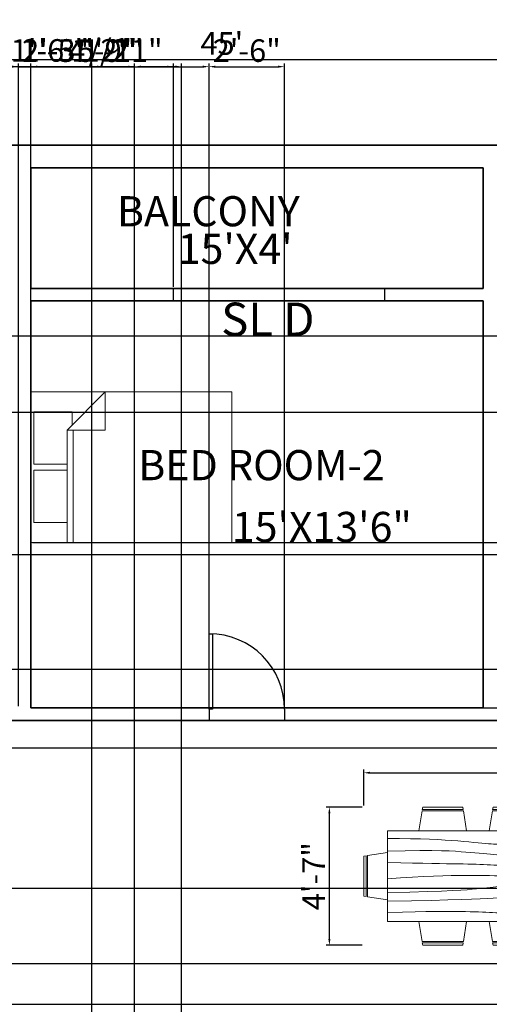
# Model space of a CAD drawing. Units: inches. Extents: x 3542 to 4275, y 1005 to 1722.
# Tile 3 of 6: x 3831 to 4018, y 1330 to 1722. Entities that reach past the tile are written whole.
import ezdxf

# ---------------------------------------------------------------- set-up
doc = ezdxf.new("R2010")
doc.units = ezdxf.units.IN
doc.layers.get('0').update_dxf_attribs({"color": 211})
for name, color, linetype, lineweight in [('A-ANNO-DIMS', 2, 'Continuous', 18), ('A-ANNO-TEXT', 7, 'Continuous', 18), ('A-AREA-IDEN', 7, 'Continuous', 25), ('A-DOOR', 3, 'Continuous', 25), ('A-FURN', 8, 'Continuous', 18), ('wall', 7, 'Continuous', 35)]:
    doc.layers.add(name, color=color, linetype=linetype, lineweight=lineweight)
doc.styles.get("Standard").update_dxf_attribs({"font": 'arial.ttf'})
doc.dimstyles.new('ISO-25', dxfattribs={"dimtxt": 9, "dimasz": 2.5, "dimexe": 1.25, "dimexo": 0.625, "dimtad": 1, "dimdec": 1, "dimlunit": 4, "dimtxsty": 'Standard', "dimcen": 2.5, "dimadec": 0, "dimazin": 0, "dimtfac": 1, "dimtdec": 1, "dimtmove": 0, "dimatfit": 3, "dimfxl": 1, "dimarcsym": 0})

# ---------------------------------------------------------------- blocks, each defined once
blk = doc.blocks.new('*U2')
for p, q in [((0, 0), (0, -6)), ((40, 0), (40, -6))]:
    blk.add_line(p, q)
blk.add_lwpolyline([(0, 0), (0, 40), (1.75, 40), (1.75, 0)], close=True)
blk.add_arc((0, 0), 40, 0, 90)
blk = doc.blocks.new('Bed - Queen')
for p, q in [((0, -80.00003), (0, 0)), ((0, 0), (59.99999, 0)), ((59.99999, 0), (59.99999, -80.00003)), ((7.99999, -1.2), (28.79998, -1.2)), ((7.99999, -14.4), (7.99999, -1.2)), ((28.79998, -1.2), (28.79998, -14.4)), ((31.19999, -1.2), (51.99999, -1.2)), ((31.19999, -14.4), (31.19999, -1.2)), ((51.99999, -1.2), (51.99999, -16.4)), ((0, -14.4), (44.8, -14.4)), ((59.99999, -29.6), (44.8, -14.4)), ((44.8, -14.4), (44.8, -29.6)), ((44.8, -16.8), (0, -16.8)), ((51.99999, -16.4), (46.79936, -16.4)), ((44.8, -29.6), (59.99999, -29.6)), ((59.99999, -80.00003), (0, -80.00003))]:
    blk.add_line(p, q)
blk = doc.blocks.new('Dining Set - 36 x 72 in.')
for p, q in [((-22, 27.5), (-22.1562, 26.50042)), ((-22, 27.5), (-6, 27.5)), ((-5.8437, 26.49966), (-6, 27.5)), ((6, 27.5), (5.8438, 26.50042)), ((6, 27.5), (22, 27.5)), ((22.1563, 26.49966), (22, 27.5)), ((-22.2343, 26.00059), (-23.4847, 17.99762)), ((-22.2304, 26), (-5.7608, 26)), ((-5.8416, 26.5), (-22.1534, 26.5)), ((-4.5152, 17.99762), (-5.7655, 25.99926)), ((5.7657, 26.00059), (4.5153, 17.99762)), ((5.7696, 26), (22.2392, 26)), ((22.1584, 26.5), (5.8466, 26.5)), ((23.4848, 17.99762), (22.2345, 25.99926)), ((36, 18), (-36, 18)), ((-36, 18), (-36, -18)), ((36, -18), (36, 18)), ((-45.5, 8), (-44.5004, 8.15617)), ((-45.5, 8), (-45.5, -8)), ((-44.5, -8.15843), (-44.5, 8.15338)), ((-44.0006, 8.23428), (-35.9976, 9.48474)), ((-44, 8.23041), (-44, -8.23915)), ((44.0006, 8.23428), (35.9976, 9.48474)), ((44, 8.23041), (44, -8.23915)), ((44.5, -8.15843), (44.5, 8.15338)), ((45.5, 8), (44.5005, 8.15617)), ((45.5, 8), (45.5, -8)), ((-44.4997, -8.15631), (-45.5, -8)), ((-35.9976, -9.48476), (-43.9993, -8.2345)), ((35.9976, -9.48476), (43.9993, -8.2345)), ((44.4997, -8.15631), (45.5, -8)), ((-36, -18), (36, -18)), ((-22.2343, -26.0006), (-23.4847, -17.99762)), ((-4.5152, -17.99762), (-5.7655, -25.99928)), ((5.7657, -26.0006), (4.5153, -17.99762)), ((23.4848, -17.99762), (22.2345, -25.99928)), ((-22.2304, -26), (-5.7608, -26)), ((-22, -27.5), (-22.1562, -26.50044)), ((-5.8416, -26.5), (-22.1534, -26.5)), ((-5.8437, -26.49967), (-6, -27.5)), ((5.7696, -26), (22.2392, -26)), ((6, -27.5), (5.8438, -26.50044)), ((22.1584, -26.5), (5.8466, -26.5)), ((22.1563, -26.49967), (22, -27.5)), ((-22, -27.5), (-6, -27.5)), ((6, -27.5), (22, -27.5))]:
    blk.add_line(p, q)
for points in [[(-36, 15), (-31.1772, 14.97754), (-26.8079, 14.91406), (-22.8538, 14.81543), (-19.276, 14.6875), (-16.0362, 14.53613), (-13.0957, 14.36718), (-10.4159, 14.18652), (-7.9583, 14), (-5.6904, 13.81315), (-3.6035, 13.63021), (-1.6954, 13.45508), (0.0365, 13.29166), (1.5945, 13.14388), (2.9811, 13.01562), (4.1988, 12.9108), (5.25, 12.83333), (6.1393, 12.78613), (6.8802, 12.76823), (7.4883, 12.77767), (7.9792, 12.8125), (8.3685, 12.87077), (8.6719, 12.95052), (8.9049, 13.0498), (9.0833, 13.16666), (9.2205, 13.29899), (9.3216, 13.44401), (9.3895, 13.59879), (9.4271, 13.76041), (9.4373, 13.92594), (9.4232, 14.09245), (9.3875, 14.257), (9.3333, 14.41666), (9.2638, 14.56917), (9.1836, 14.71484), (9.0975, 14.85465), (9.0104, 14.98958), (8.9272, 15.1206), (8.8529, 15.2487), (8.7922, 15.37483), (8.75, 15.5), (8.7305, 15.62467), (8.7344, 15.74739), (8.7617, 15.86621), (8.8125, 15.97916), (8.8867, 16.08431), (8.9844, 16.17968), (9.1055, 16.26334), (9.25, 16.33333), (9.4189, 16.38802), (9.6172, 16.42708), (9.8506, 16.45052), (10.125, 16.45833), (10.4463, 16.45052), (10.8203, 16.42708), (11.2529, 16.38802), (11.75, 16.33333), (12.3184, 16.26318), (12.9694, 16.17838), (13.7151, 16.07991), (14.5677, 15.96875), (15.5395, 15.84586), (16.6426, 15.71224), (17.8893, 15.56884), (19.2917, 15.41666), (20.859, 15.25667), (22.5879, 15.08984), (24.4721, 14.91715), (26.5052, 14.73958), (28.6809, 14.5581), (30.9929, 14.3737), (33.4347, 14.18733), (36, 14)], [(-36, 10), (-28.9766, 10.14274), (-23.1725, 10.20442), (-18.4241, 10.19775), (-14.5677, 10.13541), (-11.4399, 10.03011), (-8.877, 9.89453), (-6.7154, 9.74137), (-4.7917, 9.58333), (-2.9698, 9.43082), (-1.2246, 9.28515), (0.4415, 9.14534), (2.026, 9.01041), (3.5266, 8.87939), (4.9408, 8.7513), (6.266, 8.62516), (7.5, 8.5), (8.6411, 8.37549), (9.6914, 8.2539), (10.6538, 8.13818), (11.5312, 8.03125), (12.3267, 7.93603), (13.043, 7.85547), (13.6831, 7.79248), (14.25, 7.75), (14.7471, 7.7303), (15.1797, 7.73307), (15.5537, 7.75732), (15.875, 7.80208), (16.1494, 7.86637), (16.3828, 7.94922), (16.5811, 8.04964), (16.75, 8.16666), (16.8944, 8.29915), (17.0143, 8.44531), (17.1089, 8.60319), (17.1771, 8.77083), (17.218, 8.94629), (17.2305, 9.1276), (17.2137, 9.31282), (17.1667, 9.5), (17.0895, 9.6875), (16.987, 9.875), (16.8649, 10.0625), (16.7292, 10.25), (16.5856, 10.4375), (16.4401, 10.625), (16.2985, 10.8125), (16.1667, 11), (16.05, 11.18733), (15.9518, 11.3737), (15.8752, 11.5581), (15.8229, 11.73958), (15.798, 11.91715), (15.8034, 12.08984), (15.842, 12.25667), (15.9167, 12.41666), (16.0295, 12.56836), (16.1784, 12.70833), (16.3605, 12.83268), (16.5729, 12.9375), (16.8127, 13.01888), (17.0768, 13.07291), (17.3625, 13.0957), (17.6667, 13.08333), (17.9894, 13.03312), (18.3418, 12.94726), (18.7382, 12.82918), (19.1927, 12.68229), (19.7195, 12.51001), (20.3327, 12.31575), (21.0465, 12.10294), (21.875, 11.875), (22.8357, 11.63354), (23.959, 11.37304), (25.2786, 11.08618), (26.8282, 10.76562), (28.6414, 10.40405), (30.752, 9.99414), (33.1936, 9.52856), (36, 9)], [(-36, 5.5), (-30.7157, 5.3348), (-26.069, 5.20963), (-21.9946, 5.11767), (-18.4271, 5.05208), (-15.3009, 5.00602), (-12.5508, 4.97265), (-10.1112, 4.94515), (-7.9167, 4.91666), (-5.909, 4.88167), (-4.0586, 4.83984), (-2.3429, 4.79215), (-0.7396, 4.73958), (0.7739, 4.6831), (2.22, 4.6237), (3.6213, 4.56233), (5, 4.5), (6.373, 4.43782), (7.7344, 4.3776), (9.0723, 4.32129), (10.375, 4.27083), (11.6309, 4.22819), (12.8281, 4.19531), (13.9551, 4.17415), (15, 4.16666), (15.954, 4.17448), (16.819, 4.19791), (17.6001, 4.23698), (18.3021, 4.29166), (18.9299, 4.36198), (19.4883, 4.44791), (19.9823, 4.54948), (20.4167, 4.66666), (20.7969, 4.79899), (21.1302, 4.94401), (21.4245, 5.09879), (21.6875, 5.26041), (21.9271, 5.42594), (22.1511, 5.59245), (22.3672, 5.757), (22.5834, 5.91666), (22.8065, 6.06868), (23.0404, 6.21093), (23.2879, 6.34147), (23.5521, 6.45833), (23.8358, 6.55957), (24.142, 6.64323), (24.4735, 6.70735), (24.8334, 6.75), (25.2235, 6.76969), (25.642, 6.76692), (26.0858, 6.74267), (26.5521, 6.69791), (27.0379, 6.63362), (27.5404, 6.55078), (28.0565, 6.45036), (28.5834, 6.33333), (29.1242, 6.19987), (29.7071, 6.04687), (30.3661, 5.87044), (31.1354, 5.66666), (32.0493, 5.43164), (33.142, 5.16146), (34.4475, 4.85221), (36, 4.5)], [(-36, -1), (-30.7915, -0.6591), (-26.0195, -0.38216), (-21.6519, -0.16284), (-17.6563, 0.00521), (-14.0005, 0.12833), (-10.6523, 0.21289), (-7.5796, 0.26522), (-4.75, 0.29166), (-2.134, 0.29793), (0.2878, 0.28711), (2.5317, 0.26163), (4.6146, 0.22396), (6.5529, 0.17651), (8.3633, 0.12174), (10.0623, 0.06209), (11.6667, 0), (13.1899, -0.06201), (14.6341, -0.1211), (15.9982, -0.17432), (17.2813, -0.21875), (18.4823, -0.25147), (19.6003, -0.26953), (20.6343, -0.27002), (21.5834, -0.25), (22.4481, -0.20768), (23.2357, -0.14584), (23.9549, -0.06836), (24.6146, 0.02083), (25.2235, 0.11784), (25.7904, 0.21875), (26.3241, 0.31966), (26.8334, 0.41666), (27.3265, 0.50618), (27.8099, 0.58593), (28.2894, 0.65397), (28.7709, 0.70833), (29.2601, 0.74707), (29.763, 0.76823), (30.2855, 0.76985), (30.8334, 0.75), (31.4088, 0.70784), (31.9994, 0.64713), (32.589, 0.57275), (33.1615, 0.48958), (33.7008, 0.4025), (34.1908, 0.3164), (34.6153, 0.23616), (34.9584, 0.16666), (35.2099, 0.11165), (35.3848, 0.07031), (35.504, 0.04069), (35.5886, 0.02083), (35.6594, 0.00879), (35.7377, 0.0026), (35.8442, 0.00032), (36, 0)], [(-36, -6.5), (-27.1843, -6.31267), (-20.084, -6.1263), (-14.469, -5.9419), (-10.1094, -5.76042), (-6.7752, -5.58285), (-4.2363, -5.41016), (-2.2629, -5.24333), (-0.625, -5.08334), (0.8708, -4.93099), (2.2715, -4.78646), (3.5872, -4.64974), (4.8281, -4.52084), (6.0046, -4.39974), (7.127, -4.28646), (8.2053, -4.18099), (9.25, -4.08334), (10.2705, -3.99382), (11.2734, -3.91407), (12.2647, -3.84603), (13.25, -3.79167), (14.2354, -3.75293), (15.2266, -3.73177), (16.2295, -3.73015), (17.25, -3.75), (18.2912, -3.79248), (19.3451, -3.85547), (20.4009, -3.93604), (21.4479, -4.03125), (22.4754, -4.13819), (23.4727, -4.25391), (24.4289, -4.37549), (25.3334, -4.5), (26.1785, -4.62492), (26.9694, -4.74935), (27.7145, -4.87281), (28.4219, -4.99479), (29.1, -5.11483), (29.7572, -5.23242), (30.4016, -5.34709), (31.0417, -5.45834), (31.6837, -5.56437), (32.3262, -5.65821), (32.9658, -5.73153), (33.599, -5.77604), (34.2224, -5.78345), (34.8327, -5.74545), (35.4264, -5.65373), (36, -5.5)], [(-36, -10), (-26.4022, -9.81299), (-18.4675, -9.62891), (-11.9839, -9.45069), (-6.7396, -9.28125), (-2.5226, -9.12354), (0.8789, -8.98047), (3.6769, -8.85498), (6.0833, -8.75), (8.2767, -8.66765), (10.3021, -8.60677), (12.1712, -8.56543), (13.8958, -8.54167), (15.4876, -8.53353), (16.9583, -8.53907), (18.3197, -8.55632), (19.5834, -8.58334), (20.7616, -8.61841), (21.8685, -8.66081), (22.9188, -8.71004), (23.9271, -8.76563), (24.9081, -8.82707), (25.8763, -8.89388), (26.8465, -8.96558), (27.8334, -9.04167), (28.8474, -9.12118), (29.8828, -9.20117), (30.93, -9.27824), (31.9792, -9.34896), (33.0205, -9.40991), (34.0443, -9.45768), (35.0407, -9.48885), (36, -9.5)], [(-36, -14.5), (-30.0881, -14.33513), (-25.0332, -14.21224), (-20.7312, -14.12647), (-17.0781, -14.07292), (-13.97, -14.04671), (-11.3027, -14.04297), (-8.9724, -14.05681), (-6.875, -14.08334), (-4.9224, -14.11833), (-3.0905, -14.16016), (-1.3709, -14.20785), (0.2448, -14.26042), (1.7647, -14.3169), (3.1973, -14.3763), (4.5507, -14.43767), (5.8333, -14.5), (7.0554, -14.5621), (8.235, -14.62175), (9.3922, -14.67652), (10.5469, -14.72396), (11.7192, -14.76164), (12.929, -14.78711), (14.1965, -14.79794), (15.5417, -14.79167), (16.9933, -14.76424), (18.6152, -14.70508), (20.4804, -14.60197), (22.6615, -14.44271), (25.2312, -14.21509), (28.2624, -13.9069), (31.8277, -13.50594), (36, -13)]]:
    blk.add_lwpolyline(points)
blk = doc.blocks.new('*D12')
at = {"layer": 'A-ANNO-DIMS', "color": 0, "lineweight": -2, "transparency": 16777216}
for p, q in [((3641.89, 1673.05), (3641.89, 1707.82)), ((3644.39, 1706.57), (4179.39, 1706.57)), ((4181.89, 1673.05), (4181.89, 1707.82))]:
    blk.add_line(p, q, dxfattribs=at)
at = {"layer": 'A-ANNO-DIMS', "color": 0, "transparency": 16777216}
for points in [[(3644.39, 1706.99), (3644.39, 1706.16), (3641.89, 1706.57)], [(4179.39, 1706.99), (4179.39, 1706.16), (4181.89, 1706.57)]]:
    blk.add_solid(points, dxfattribs=at)
at = {"layer": 'Defpoints', "color": 0, "transparency": 16777216}
for p in [(4181.89, 1706.57), (3641.89, 1672.43), (4181.89, 1672.43)]:
    blk.add_point(p, dxfattribs=at)
at = {"layer": 'A-ANNO-DIMS', "color": 0, "transparency": 16777216, "insert": (3911.89, 1711.77), "char_height": 9, "attachment_point": 5}
blk.add_mtext("45'", dxfattribs=at)
blk = doc.blocks.new('DOOR-SLIDING-84IN')
blk.add_lwpolyline([(0, 0), (0, 5), (84, 5), (84, 0)], close=True)
blk = doc.blocks.new('*D31')
at = {"layer": 'A-ANNO-DIMS', "color": 0, "lineweight": -2, "transparency": 16777216}
for p, q in [((3968.37, 1409.56), (3968.37, 1423.84)), ((4059.37, 1409.56), (4059.37, 1423.84)), ((3970.87, 1422.59), (4056.87, 1422.59)), ((4059.37, 1422.59), (4162.04, 1422.59))]:
    blk.add_line(p, q, dxfattribs=at)
at = {"layer": 'A-ANNO-DIMS', "color": 0, "transparency": 16777216}
for points in [[(3970.87, 1423.01), (3970.87, 1422.17), (3968.37, 1422.59)], [(4056.87, 1423.01), (4056.87, 1422.17), (4059.37, 1422.59)]]:
    blk.add_solid(points, dxfattribs=at)
at = {"layer": 'Defpoints', "color": 0, "transparency": 16777216}
for p in [(4059.37, 1422.59), (3968.37, 1408.94), (4059.37, 1408.94)]:
    blk.add_point(p, dxfattribs=at)
at = {"layer": 'A-ANNO-DIMS', "color": 0, "transparency": 16777216, "insert": (4111.95, 1427.87), "char_height": 9, "attachment_point": 5}
blk.add_mtext('DINING SET 7\'-7"', dxfattribs=at)
blk = doc.blocks.new('*D32')
at = {"layer": 'A-ANNO-DIMS', "color": 0, "lineweight": -2, "transparency": 16777216}
for p, q in [((3967.74, 1408.94), (3953.47, 1408.94)), ((3954.72, 1356.44), (3954.72, 1406.44)), ((3967.74, 1353.94), (3953.47, 1353.94))]:
    blk.add_line(p, q, dxfattribs=at)
at = {"layer": 'A-ANNO-DIMS', "color": 0, "transparency": 16777216}
for points in [[(3954.3, 1406.44), (3955.14, 1406.44), (3954.72, 1408.94)], [(3954.3, 1356.44), (3955.14, 1356.44), (3954.72, 1353.94)]]:
    blk.add_solid(points, dxfattribs=at)
at = {"layer": 'Defpoints', "color": 0, "transparency": 16777216}
for p in [(3954.72, 1408.94), (3968.37, 1408.94), (3968.37, 1353.94)]:
    blk.add_point(p, dxfattribs=at)
at = {"layer": 'A-ANNO-DIMS', "color": 0, "transparency": 16777216, "insert": (3949.59, 1381.44), "char_height": 9, "attachment_point": 5, "rotation": 90}
blk.add_mtext('4\'-7"', dxfattribs=at)
blk = doc.blocks.new('*D43')
at = {"layer": 'A-ANNO-DIMS', "color": 0, "lineweight": -2, "transparency": 16777216}
for p, q in [((3835.89, 1616.05), (3835.89, 1704.93)), ((3838.39, 1703.68), (3890.15, 1703.68)), ((3892.65, 1616.05), (3892.65, 1704.93))]:
    blk.add_line(p, q, dxfattribs=at)
at = {"layer": 'A-ANNO-DIMS', "color": 0, "transparency": 16777216}
for points in [[(3838.39, 1704.09), (3838.39, 1703.26), (3835.89, 1703.68)], [(3890.15, 1704.09), (3890.15, 1703.26), (3892.65, 1703.68)]]:
    blk.add_solid(points, dxfattribs=at)
at = {"layer": 'Defpoints', "color": 0, "transparency": 16777216}
for p in [(3892.65, 1703.68), (3835.89, 1615.43), (3892.65, 1615.43)]:
    blk.add_point(p, dxfattribs=at)
at = {"layer": 'A-ANNO-DIMS', "color": 0, "transparency": 16777216, "insert": (3864.27, 1708.9), "char_height": 9, "attachment_point": 5}
blk.add_mtext('4\'-9"', dxfattribs=at)
blk = doc.blocks.new('*D46')
at = {"layer": 'A-ANNO-DIMS', "color": 0, "lineweight": -2, "transparency": 16777216}
for p, q in [((3803.24, 1444.05), (3803.24, 1704.93)), ((3805.74, 1703.68), (3828.39, 1703.68)), ((3830.89, 1449.05), (3830.89, 1704.93)), ((3830.89, 1703.68), (3879.69, 1703.68))]:
    blk.add_line(p, q, dxfattribs=at)
at = {"layer": 'A-ANNO-DIMS', "color": 0, "transparency": 16777216}
for points in [[(3805.74, 1704.09), (3805.74, 1703.26), (3803.24, 1703.68)], [(3828.39, 1704.09), (3828.39, 1703.26), (3830.89, 1703.68)]]:
    blk.add_solid(points, dxfattribs=at)
at = {"layer": 'Defpoints', "color": 0, "transparency": 16777216}
for p in [(3830.89, 1703.68), (3830.89, 1448.43), (3803.24, 1443.43)]:
    blk.add_point(p, dxfattribs=at)
at = {"layer": 'A-ANNO-DIMS', "color": 0, "transparency": 16777216, "insert": (3856.54, 1708.96), "char_height": 9, "attachment_point": 5}
blk.add_mtext('2\'-3 1/2"', dxfattribs=at)
blk = doc.blocks.new('*D47')
at = {"layer": 'A-ANNO-DIMS', "color": 0, "lineweight": -2, "transparency": 16777216}
for p, q in [((3835.89, 1449.05), (3835.89, 1704.93)), ((3838.39, 1703.68), (3904.32, 1703.68)), ((3906.82, 1448.55), (3906.82, 1704.93))]:
    blk.add_line(p, q, dxfattribs=at)
at = {"layer": 'A-ANNO-DIMS', "color": 0, "transparency": 16777216}
for points in [[(3838.39, 1704.09), (3838.39, 1703.26), (3835.89, 1703.68)], [(3904.32, 1704.09), (3904.32, 1703.26), (3906.82, 1703.68)]]:
    blk.add_solid(points, dxfattribs=at)
at = {"layer": 'Defpoints', "color": 0, "transparency": 16777216}
for p in [(3906.82, 1703.68), (3835.89, 1448.43), (3906.82, 1447.93)]:
    blk.add_point(p, dxfattribs=at)
at = {"layer": 'A-ANNO-DIMS', "color": 0, "transparency": 16777216, "insert": (3871.35, 1708.9), "char_height": 9, "attachment_point": 5}
blk.add_mtext('5\'-11"', dxfattribs=at)
blk = doc.blocks.new('*D48')
at = {"layer": 'A-ANNO-DIMS', "color": 0, "lineweight": -2, "transparency": 16777216}
for p, q in [((3906.82, 1448.55), (3906.82, 1704.93)), ((3909.32, 1703.68), (3934.32, 1703.68)), ((3936.82, 1448.55), (3936.82, 1704.93))]:
    blk.add_line(p, q, dxfattribs=at)
at = {"layer": 'A-ANNO-DIMS', "color": 0, "transparency": 16777216}
for points in [[(3909.32, 1704.09), (3909.32, 1703.26), (3906.82, 1703.68)], [(3934.32, 1704.09), (3934.32, 1703.26), (3936.82, 1703.68)]]:
    blk.add_solid(points, dxfattribs=at)
at = {"layer": 'Defpoints', "color": 0, "transparency": 16777216}
for p in [(3936.82, 1703.68), (3906.82, 1447.93), (3936.82, 1447.93)]:
    blk.add_point(p, dxfattribs=at)
at = {"layer": 'A-ANNO-DIMS', "color": 0, "transparency": 16777216, "insert": (3921.82, 1708.9), "char_height": 9, "attachment_point": 5}
blk.add_mtext('2\'-6"', dxfattribs=at)
blk = doc.blocks.new('*D54')
at = {"layer": 'A-ANNO-DIMS', "color": 0, "lineweight": -2, "transparency": 16777216}
for p, q in [((4047.2, 1596.46), (3559.02, 1596.46)), ((3560.27, 1593.96), (3560.27, 1568.52)), ((4047.2, 1566.02), (3559.02, 1566.02)), ((3560.27, 1566.02), (3560.27, 1517.22))]:
    blk.add_line(p, q, dxfattribs=at)
at = {"layer": 'A-ANNO-DIMS', "color": 0, "transparency": 16777216}
for points in [[(3559.85, 1593.96), (3560.69, 1593.96), (3560.27, 1596.46)], [(3559.85, 1568.52), (3560.69, 1568.52), (3560.27, 1566.02)]]:
    blk.add_solid(points, dxfattribs=at)
at = {"layer": 'Defpoints', "color": 0, "transparency": 16777216}
for p in [(4047.82, 1596.46), (3560.27, 1566.02), (4047.82, 1566.02)]:
    blk.add_point(p, dxfattribs=at)
at = {"layer": 'A-ANNO-DIMS', "color": 0, "transparency": 16777216, "insert": (3554.99, 1540.37), "char_height": 9, "attachment_point": 5, "rotation": 90}
blk.add_mtext('2\'-6 1/2"', dxfattribs=at)
blk = doc.blocks.new('*D55')
at = {"layer": 'A-ANNO-DIMS', "color": 0, "lineweight": -2, "transparency": 16777216}
for p, q in [((3560.27, 1509.3), (3560.27, 1557.94)), ((4047.2, 1509.3), (3559.02, 1509.3)), ((3560.27, 1466.15), (3560.27, 1506.8)), ((4047.2, 1463.65), (3559.02, 1463.65))]:
    blk.add_line(p, q, dxfattribs=at)
at = {"layer": 'A-ANNO-DIMS', "color": 0, "transparency": 16777216}
for points in [[(3559.85, 1506.8), (3560.69, 1506.8), (3560.27, 1509.3)], [(3559.85, 1466.15), (3560.69, 1466.15), (3560.27, 1463.65)]]:
    blk.add_solid(points, dxfattribs=at)
at = {"layer": 'Defpoints', "color": 0, "transparency": 16777216}
for p in [(3560.27, 1509.3), (4047.82, 1509.3), (4047.82, 1463.65)]:
    blk.add_point(p, dxfattribs=at)
at = {"layer": 'A-ANNO-DIMS', "color": 0, "transparency": 16777216, "insert": (3554.99, 1534.87), "char_height": 9, "attachment_point": 5, "rotation": 90}
blk.add_mtext('3\'-9 1/2"', dxfattribs=at)
blk = doc.blocks.new('*D60')
at = {"layer": 'A-ANNO-DIMS', "color": 0, "lineweight": -2, "transparency": 16777216}
for p, q in [((3860.16, 1703.68), (3833.33, 1703.68)), ((3860.16, 1207.47), (3860.16, 1704.93)), ((3874.66, 1703.68), (3862.66, 1703.68)), ((3877.16, 1207.47), (3877.16, 1704.93))]:
    blk.add_line(p, q, dxfattribs=at)
at = {"layer": 'A-ANNO-DIMS', "color": 0, "transparency": 16777216}
for points in [[(3862.66, 1704.09), (3862.66, 1703.26), (3860.16, 1703.68)], [(3874.66, 1704.09), (3874.66, 1703.26), (3877.16, 1703.68)]]:
    blk.add_solid(points, dxfattribs=at)
at = {"layer": 'Defpoints', "color": 0, "transparency": 16777216}
for p in [(3860.16, 1703.68), (3860.16, 1206.85), (3877.16, 1206.85)]:
    blk.add_point(p, dxfattribs=at)
at = {"layer": 'A-ANNO-DIMS', "color": 0, "transparency": 16777216, "insert": (3845.5, 1708.9), "char_height": 9, "attachment_point": 5}
blk.add_mtext('1\'-5"', dxfattribs=at)
blk = doc.blocks.new('*D61')
at = {"layer": 'A-ANNO-DIMS', "color": 0, "lineweight": -2, "transparency": 16777216}
for p, q in [((3877.16, 1703.68), (3829.36, 1703.68)), ((3877.16, 1207.47), (3877.16, 1704.93)), ((3893.39, 1703.68), (3879.66, 1703.68)), ((3895.89, 1207.05), (3895.89, 1704.93))]:
    blk.add_line(p, q, dxfattribs=at)
at = {"layer": 'A-ANNO-DIMS', "color": 0, "transparency": 16777216}
for points in [[(3879.66, 1704.09), (3879.66, 1703.26), (3877.16, 1703.68)], [(3893.39, 1704.09), (3893.39, 1703.26), (3895.89, 1703.68)]]:
    blk.add_solid(points, dxfattribs=at)
at = {"layer": 'Defpoints', "color": 0, "transparency": 16777216}
for p in [(3877.16, 1703.68), (3877.16, 1206.85), (3895.89, 1206.43)]:
    blk.add_point(p, dxfattribs=at)
at = {"layer": 'A-ANNO-DIMS', "color": 0, "transparency": 16777216, "insert": (3852.01, 1708.96), "char_height": 9, "attachment_point": 5}
blk.add_mtext('1\'-6 1/2"', dxfattribs=at)
blk = doc.blocks.new('*D64')
at = {"layer": 'A-ANNO-DIMS', "color": 0, "lineweight": -2, "transparency": 16777216}
for p, q in [((3741.01, 1376.72), (4214.39, 1376.72)), ((4213.14, 1374.22), (4213.14, 1349.22)), ((3741.01, 1346.72), (4214.39, 1346.72))]:
    blk.add_line(p, q, dxfattribs=at)
at = {"layer": 'A-ANNO-DIMS', "color": 0, "transparency": 16777216}
for points in [[(4212.72, 1374.22), (4213.56, 1374.22), (4213.14, 1376.72)], [(4212.72, 1349.22), (4213.56, 1349.22), (4213.14, 1346.72)]]:
    blk.add_solid(points, dxfattribs=at)
at = {"layer": 'Defpoints', "color": 0, "transparency": 16777216}
for p in [(3740.38, 1376.72), (3740.38, 1346.72), (4213.14, 1346.72)]:
    blk.add_point(p, dxfattribs=at)
at = {"layer": 'A-ANNO-DIMS', "color": 0, "transparency": 16777216, "insert": (4207.92, 1361.72), "char_height": 9, "attachment_point": 5, "rotation": 90}
blk.add_mtext('2\'-6"', dxfattribs=at)
blk = doc.blocks.new('*D66')
at = {"layer": 'A-ANNO-DIMS', "color": 0, "lineweight": -2, "transparency": 16777216}
for p, q in [((3735.51, 1443.43), (4214.39, 1443.43)), ((4213.14, 1440.93), (4213.14, 1435.03)), ((3735.95, 1432.53), (4214.39, 1432.53)), ((4213.14, 1432.53), (4213.14, 1397.86))]:
    blk.add_line(p, q, dxfattribs=at)
at = {"layer": 'A-ANNO-DIMS', "color": 0, "transparency": 16777216}
for points in [[(4212.72, 1440.93), (4213.56, 1440.93), (4213.14, 1443.43)], [(4212.72, 1435.03), (4213.56, 1435.03), (4213.14, 1432.53)]]:
    blk.add_solid(points, dxfattribs=at)
at = {"layer": 'Defpoints', "color": 0, "transparency": 16777216}
for p in [(3734.89, 1443.43), (3735.32, 1432.53), (4213.14, 1432.53)]:
    blk.add_point(p, dxfattribs=at)
at = {"layer": 'A-ANNO-DIMS', "color": 0, "transparency": 16777216, "insert": (4207.92, 1413.94), "char_height": 9, "attachment_point": 5, "rotation": 90}
blk.add_mtext('0\'-11"', dxfattribs=at)
blk = doc.blocks.new('*D67')
at = {"layer": 'A-ANNO-DIMS', "color": 0, "lineweight": -2, "transparency": 16777216}
for p, q in [((4213.14, 1346.72), (4213.14, 1394.52)), ((3741.01, 1346.72), (4214.39, 1346.72)), ((4213.14, 1332.93), (4213.14, 1344.22)), ((3740.51, 1330.43), (4214.39, 1330.43))]:
    blk.add_line(p, q, dxfattribs=at)
at = {"layer": 'A-ANNO-DIMS', "color": 0, "transparency": 16777216}
for points in [[(4212.72, 1344.22), (4213.56, 1344.22), (4213.14, 1346.72)], [(4212.72, 1332.93), (4213.56, 1332.93), (4213.14, 1330.43)]]:
    blk.add_solid(points, dxfattribs=at)
at = {"layer": 'Defpoints', "color": 0, "transparency": 16777216}
for p in [(3740.38, 1346.72), (4213.14, 1346.72), (3739.89, 1330.43)]:
    blk.add_point(p, dxfattribs=at)
at = {"layer": 'A-ANNO-DIMS', "color": 0, "transparency": 16777216, "insert": (4207.86, 1371.87), "char_height": 9, "attachment_point": 5, "rotation": 90}
blk.add_mtext('1\'-4 1/2"', dxfattribs=at)
blk = doc.blocks.new('*D73')
at = {"layer": 'A-ANNO-DIMS', "color": 0, "lineweight": -2, "transparency": 16777216}
for p, q in [((3836.51, 1514.23), (4214.39, 1514.23)), ((4213.14, 1450.93), (4213.14, 1511.73)), ((3836.51, 1448.43), (4214.39, 1448.43))]:
    blk.add_line(p, q, dxfattribs=at)
at = {"layer": 'A-ANNO-DIMS', "color": 0, "transparency": 16777216}
for points in [[(4212.72, 1511.73), (4213.56, 1511.73), (4213.14, 1514.23)], [(4212.72, 1450.93), (4213.56, 1450.93), (4213.14, 1448.43)]]:
    blk.add_solid(points, dxfattribs=at)
at = {"layer": 'Defpoints', "color": 0, "transparency": 16777216}
for p in [(3835.89, 1514.23), (4213.14, 1514.23), (3835.89, 1448.43)]:
    blk.add_point(p, dxfattribs=at)
at = {"layer": 'A-ANNO-DIMS', "color": 0, "transparency": 16777216, "insert": (4207.92, 1481.33), "char_height": 9, "attachment_point": 5, "rotation": 90}
blk.add_mtext('5\'-6"', dxfattribs=at)

msp = doc.modelspace()

# ---------------------------------------------------------------- linework, layer by layer
at = {"layer": 'wall'}
for p, q in [((3641.89, 1672.43), (4181.89, 1672.43)), ((3835.89, 1663.43), (4015.89, 1663.43)), ((3835.89, 1615.43), (3835.89, 1663.43)), ((4015.89, 1615.43), (4015.89, 1663.43)), ((3835.89, 1615.43), (4015.89, 1615.43)), ((3835.89, 1448.43), (3835.89, 1610.43)), ((3835.89, 1610.43), (4015.89, 1610.43)), ((4015.89, 1448.43), (4015.89, 1610.43)), ((3835.89, 1448.43), (4015.89, 1448.43)), ((3739.89, 1443.43), (4058.5, 1443.43))]:
    msp.add_line(p, q, dxfattribs=at)

# ---------------------------------------------------------------- block references
at = {"layer": 'A-DOOR'}
msp.add_blockref('DOOR-SLIDING-84IN', (3892.65, 1610.43), dxfattribs=at)
at = {"layer": 'A-DOOR', "xscale": 0.75, "yscale": 0.75, "zscale": 0.75}
msp.add_blockref('*U2', (3906.82, 1447.93), dxfattribs=at)
at = {"layer": 'A-FURN', "rotation": 90}
msp.add_blockref('Bed - Queen', (3835.89, 1514.23), dxfattribs=at)
at = {"layer": 'A-FURN'}
msp.add_blockref('Dining Set - 36 x 72 in.', (4013.87, 1381.44), dxfattribs=at)

# ---------------------------------------------------------------- texts
at = {"layer": 'A-ANNO-TEXT'}
msp.add_text('SL D', height=13.276, dxfattribs=at).set_placement((3911.64, 1596.48))
at = {"layer": 'A-AREA-IDEN'}
for s, p in [('BALCONY', (3870.15, 1640.13)), ("15'X4'", (3894.35, 1625.16)), ('BED ROOM-2', (3878.63, 1539.06)), ('15\'X13\'6"', (3915.89, 1514.45))]:
    msp.add_text(s, height=12, dxfattribs=at).set_placement(p)

# ---------------------------------------------------------------- dimensions: what is measured, and where the dimension line sits
at = {"layer": 'A-ANNO-DIMS'}
for base, p1, p2, override, picture, middle in [((3830.8894, 1703.6779), (3803.2386, 1443.4279), (3830.8894, 1448.4279), {"dimdec": 1, "dimlfac": 1, "dimrnd": 0, "dimzin": 1, "dimdsep": 46, "dimlunit": 4, "dimfrac": 2}, '*D46', (3856.5389, 1708.9594)), ((3877.16, 1703.68), (3895.89, 1206.43), (3877.16, 1206.85), {"dimdec": 1, "dimlfac": 1, "dimrnd": 0, "dimzin": 1, "dimdsep": 46, "dimlunit": 4, "dimfrac": 2}, '*D61', (3852.01, 1708.96)), ((4181.89, 1706.57), (3641.89, 1672.43), (4181.89, 1672.43), {"dimclrd": 0, "dimclre": 0, "dimclrt": 0}, '*D12', (3911.89, 1711.77)), ((3860.16, 1703.68), (3877.16, 1206.85), (3860.16, 1206.85), {"dimdec": 1, "dimlfac": 1, "dimrnd": 0, "dimzin": 1, "dimdsep": 46, "dimlunit": 4, "dimfrac": 2}, '*D60', (3845.5, 1708.9)), ((3892.65, 1703.68), (3835.89, 1615.43), (3892.65, 1615.43), {"dimdec": 1, "dimlfac": 1, "dimrnd": 0, "dimzin": 1, "dimdsep": 46, "dimlunit": 4, "dimfrac": 2}, '*D43', (3864.27, 1708.9)), ((3906.82, 1703.68), (3835.89, 1448.43), (3906.82, 1447.93), {"dimdec": 1, "dimlfac": 1, "dimrnd": 0, "dimzin": 1, "dimdsep": 46, "dimlunit": 4, "dimfrac": 2}, '*D47', (3871.35, 1708.9)), ((3936.82, 1703.68), (3906.82, 1447.93), (3936.82, 1447.93), {"dimdec": 1, "dimlfac": 1, "dimrnd": 0, "dimzin": 1, "dimdsep": 46, "dimlunit": 4, "dimfrac": 2}, '*D48', (3921.82, 1708.9))]:
    dim = msp.add_linear_dim(base=base, p1=p1, p2=p2, dimstyle='ISO-25', override=override, dxfattribs=at)
    dim.commit()
    dim.dimension.update_dxf_attribs({"geometry": picture, "text_midpoint": middle})
for base, p1, p2, picture, middle in [((3560.27, 1566.02), (4047.82, 1596.46), (4047.82, 1566.02), '*D54', (3554.99, 1540.37)), ((3560.2694, 1509.3049), (4047.8245, 1463.6541), (4047.8245, 1509.3049), '*D55', (3554.9879, 1534.8747)), ((4213.14, 1514.23), (3835.89, 1448.43), (3835.89, 1514.23), '*D73', (4207.92, 1481.33)), ((4213.14, 1432.53), (3734.89, 1443.43), (3735.32, 1432.53), '*D66', (4207.92, 1413.94)), ((3954.72, 1408.94), (3968.37, 1353.94), (3968.37, 1408.94), '*D32', (3949.59, 1381.44)), ((4213.14, 1346.72), (3739.89, 1330.43), (3740.38, 1346.72), '*D67', (4207.86, 1371.87)), ((4213.14, 1346.72), (3740.38, 1376.72), (3740.38, 1346.72), '*D64', (4207.92, 1361.72))]:
    dim = msp.add_linear_dim(base=base, p1=p1, p2=p2, angle=90, dimstyle='ISO-25', override={"dimdec": 1, "dimlfac": 1, "dimrnd": 0, "dimzin": 1, "dimdsep": 46, "dimlunit": 4, "dimfrac": 2}, dxfattribs=at)
    dim.commit()
    dim.dimension.update_dxf_attribs({"geometry": picture, "text_midpoint": middle})
dim = msp.add_linear_dim(base=(4059.37, 1422.59), p1=(3968.37, 1408.94), p2=(4059.37, 1408.94), text='DINING SET <>', dimstyle='ISO-25', override={"dimdec": 1, "dimlfac": 1, "dimrnd": 0, "dimzin": 1, "dimdsep": 46, "dimlunit": 4, "dimfrac": 2}, dxfattribs=at)
dim.commit()
dim.dimension.update_dxf_attribs({"geometry": '*D31', "text_midpoint": (4111.95, 1427.87)})

doc.saveas('drawing.dxf')
